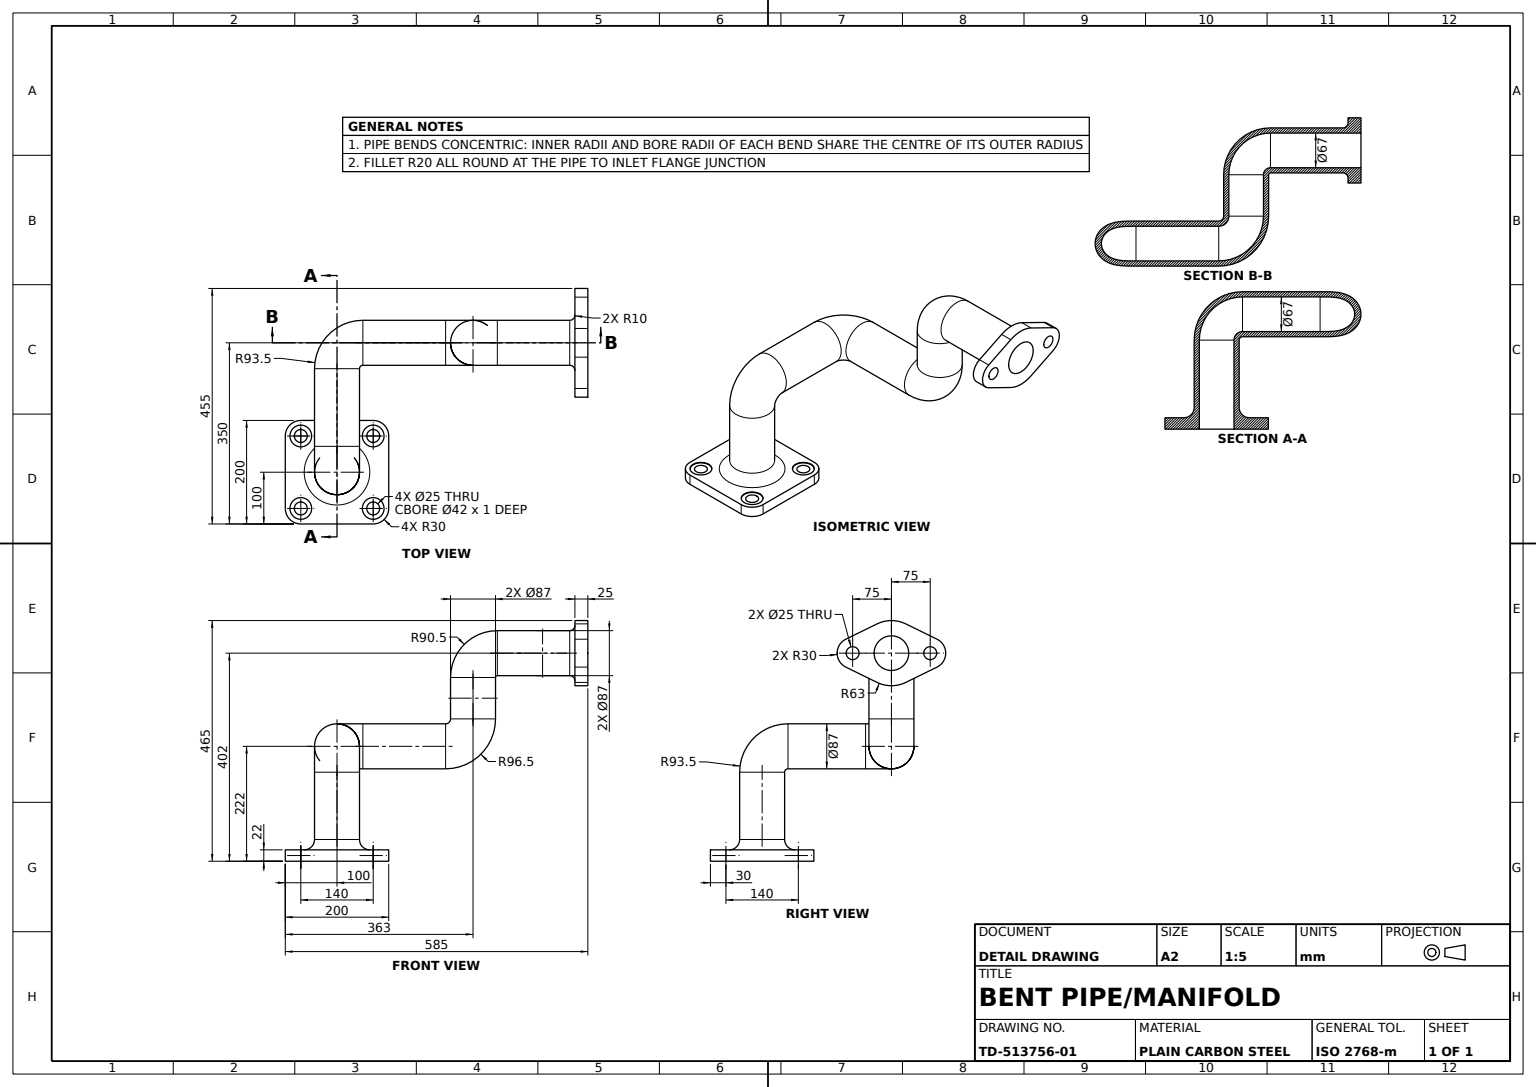
SolidWorks part; units mm, degrees
material "Plain Carbon Steel"
ref_plane "Front Plane" through (0, 0, 0) normal (0, 0, 1) x (1, 0, 0)
ref_plane "Top Plane" through (0, 0, 0) normal (0, 1, 0) x (1, 0, 0)
ref_plane "Right Plane" through (0, 0, 0) normal (1, 0, 0) x (0, 0, -1)
sketch "Inlet Flange Sketch" plane through (0, 0, 0) normal (0, 1, 0) x (1, 0, 0)
  line L1 (-70, 100) -> (70, 100)
  line L2 (-100, 70) -> (-100, -70)
  line L3 (-70, -100) -> (70, -100)
  line L4 (100, 70) -> (100, -70)
  line L5 (-100, 100) -> (100, -100) construction
  line L6 (-100, -100) -> (100, 100) construction
  arc A0 (70, -100) -> (100, -70) centre (70, -70) ccw
  arc A1 (-100, -70) -> (-70, -100) centre (-70, -70) ccw
  arc A2 (-70, 100) -> (-100, 70) centre (-70, 70) ccw
  arc A3 (70, 100) -> (100, 70) centre (70, 70) cw
  circle A4 centre (-70, 70) radius 12.5
  circle A5 centre (70, 70) radius 12.5
  circle A6 centre (70, -70) radius 12.5
  circle A7 centre (-70, -70) radius 12.5
  point P0 (0, 0)
  dimension "D2" = 30
  dimension "D3" = 25
  dimension "D4" = 25
  dimension "D5" = 25
  dimension "D6" = 25
  dimension "D1" = 200
extrude "Inlet Flange 200x200x22" add sketch "Inlet Flange Sketch" along normal blind 22
sketch "Bolt Spotface Sketch" plane through (0, 22, 0) normal (0, 1, 0) x (1, 0, 0)
  circle A0 centre (-70, 70) radius 21
  circle A1 centre (70, 70) radius 21
  circle A2 centre (70, -70) radius 21
  circle A3 centre (-70, -70) radius 21
  dimension "D1" = 42
  dimension "D2" = 42
  dimension "D3" = 42
  dimension "D4" = 42
extrude "Bolt Spotfaces 4xØ42" cut sketch "Bolt Spotface Sketch" against normal blind 1
sketch "Inlet Bore Sketch" plane through (0, 22, 0) normal (0, 1, 0) x (1, 0, 0)
  circle A0 centre (0, 0) radius 33.5
  dimension "D1" = 67
extrude "Inlet Bore Ø67" cut sketch "Inlet Bore Sketch" against normal blind 25
ref_plane "Plane1" through (400, 0, 0) normal (1, 0, 0) x (0, 0, -1)
sketch "Pipe Section 1 Profile" plane through (0, 22, 0) normal (0, 1, 0) x (1, 0, 0)
  circle A0 centre (0, 0) radius 33.5
  dimension "D1" = 67
sketch "Pipe Section 1 Path" plane through (0, 0, 0) normal (1, 0, 0) x (0, 0, -1)
  line L0 (0, 22) -> (0, 172)
  line L1 (33.5, 22) -> (-33.5, 22) construction
  line L2 (50, 222) -> (180, 222)
  arc A0 (0, 172) -> (50, 222) centre (50, 172) cw
  point P8 (0, 222)
  dimension "D3" = 50
  dimension "D1" = 200
  dimension "D2" = 180
ref_plane "Plane3" through (0, 0, -180) normal (0, 0, 1) x (1, 0, 0)
ref_plane "Plane4" through (0, 222, 0) normal (0, 1, 0) x (1, 0, 0)
sweep "Pipe Section 1" add profiles "Pipe Section 1 Profile" path "Pipe Section 1 Path" parameters "D1"=10
ref_plane "Pipe Section 2 Plane" through (0, 225, 0) normal (0, 1, 0) x (1, 0, 0)
sketch "Pipe Section 2 Path" plane through (0, 225, 0) normal (0, 1, 0) x (1, 0, 0)
  line L0 (0, 50) -> (0, 200)
  line L1 (-43.5, 50) -> (43.5, 50) construction
  line L2 (50, 250) -> (200, 250)
  arc A0 (0, 200) -> (50, 250) centre (50, 200) cw
  point P8 (0, 250)
  dimension "D3" = 50
  dimension "D1" = 200
  dimension "D2" = 200
sketch "Pipe Section 2 Profile" plane through (0, 0, -180) normal (0, 0, -1) x (-1, 0, 0)
  circle A0 centre (0, 222) radius 33.5
  dimension "D1" = 67
sweep "Pipe Section 2" add profiles "Pipe Section 2 Profile" path "Pipe Section 2 Path" parameters "D1"=10
ref_plane "S-Bend Plane" through (0, 0, -250) normal (0, 0, 1) x (1, 0, 0)
sketch "S-Bend Path" plane through (0, 0, -250) normal (0, 0, 1) x (1, 0, 0)
  line L0 (200, 225) -> (210, 225)
  line L1 (50, 225) -> (200, 225) construction
  line L2 (260, 275) -> (260, 355)
  line L3 (310, 405) -> (460, 405)
  arc A0 (260, 355) -> (310, 405) centre (310, 355) cw
  arc A1 (210, 225) -> (260, 275) centre (210, 275) ccw
  point P11 (260, 225)
  dimension "D2" = 50
  dimension "D1" = 60
  dimension "D3" = 80
  dimension "D4" = 200
  dimension "D5" = 200
sketch "S-Bend Profile" plane through (200, 0, 0) normal (1, 0, 0) x (0, 0, -1)
  circle A1 centre (250, 222) radius 33.5
  dimension "D1" = 67
sweep "S-Bend Pipe Section" add profiles "S-Bend Profile" path "S-Bend Path" parameters "D1"=10
sketch "Outlet Flange Sketch" plane through (460, 0, 0) normal (1, 0, 0) x (0, 0, -1)
  line L0 (222.28, 458.5739) -> (161.8, 428.9399)
  line L1 (161.8, 375.0601) -> (222.28, 345.4261)
  line L2 (277.72, 458.5739) -> (338.2, 428.9399)
  line L3 (277.72, 345.4261) -> (338.2, 375.0601)
  circle A0 centre (250, 402) radius 33.5
  arc A2 (338.2, 375.0601) -> (338.2, 428.9399) centre (325, 402) ccw
  circle A3 centre (325, 402) radius 12.5
  arc A4 (161.8, 428.9399) -> (161.8, 375.0601) centre (175, 402) ccw
  circle A5 centre (175, 402) radius 12.5
  arc A6 (222.28, 345.4261) -> (277.72, 345.4261) centre (250, 402) ccw
  arc A8 (277.72, 458.5739) -> (222.28, 458.5739) centre (250, 402) ccw
  dimension "D1" = 26.9399
  dimension "D2" = 67
  dimension "D3" = 60
  dimension "D4" = 25
  dimension "D5" = 60
  dimension "D6" = 25
  dimension "D7" = 75
  dimension "D8" = 75
  dimension "D9" = 56.5739
  dimension "D10" = 56.5739
  dimension "D11" = 56.5739
  dimension "D12" = 26.9399
  dimension "D13" = 29.6339
extrude "Outlet Flange" add sketch "Outlet Flange Sketch" along normal blind 25
fillet "Inlet Flange Fillet R20" radius 20 1 edges at (0, 22, 43.5)
fillet "Outlet Fillet R10" radius 10 1 edges at (460, 402, -293.5)
